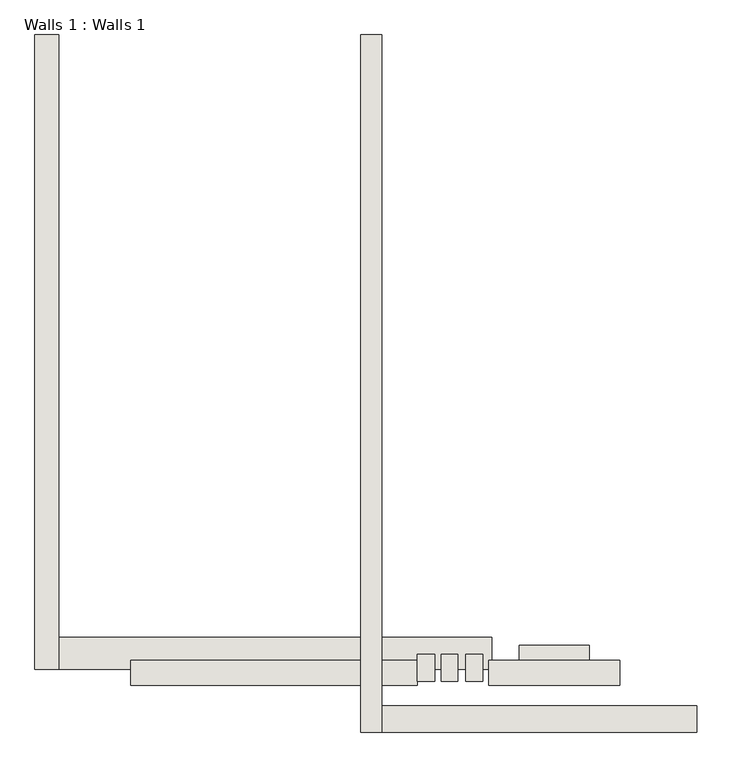
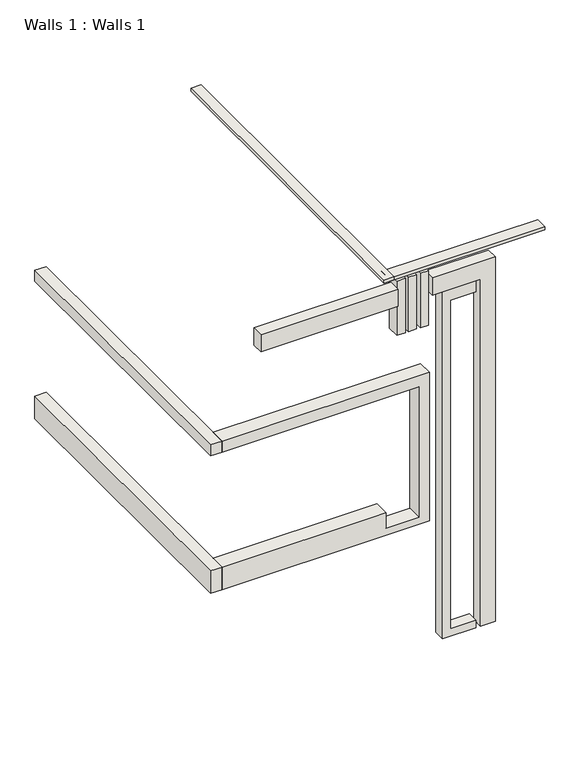
"""IFC4 building model written with IfcOpenShell, lengths in millimetres: wall geometry, Walls 1 : Walls 1."""

from ifc_helpers import new_model, si_unit, frame, origin, place, context, project, spatial, polyline, outline, extrude, source, transform, mapped, element, save


def walls_1_walls_1_d3114a13(model_context):
    return source(origin(), model_context, "Body", "SweptSolid", [
        extrude(outline(polyline([(-3875.3528989, 2861.5277146), (-3875.3528989, 11743.1483979), (-3610.0128864, 11743.1483979), (-3610.0128864, 2861.5277146), (-3875.3528989, 2861.5277146)])), frame((0.0, 0.0, 11198.7570873), z_axis=(0.0, 0.0, 1.0), x_axis=(1.0, 0.0, 0.0)), (0.0, 0.0, 1.0), 78.8429127),
        extrude(outline(polyline([(399.1874342, 2861.5277146), (-3753.7125658, 2861.5277146), (-3753.7125658, 3200.3867317), (399.1874342, 3200.3867317), (399.1874342, 2861.5277146)])), frame((0.0, 0.0, 11198.7570873), z_axis=(0.0, 0.0, 1.0), x_axis=(1.0, 0.0, 0.0)), (0.0, 0.0, 1.0), 78.8429127),
        extrude(outline(polyline([(-8020.9125658, 3665.9483979), (-8020.9125658, 11743.1483979), (-7716.1125658, 11743.1483979), (-7716.1125658, 3665.9483979), (-8020.9125658, 3665.9483979)])), frame((0.0, 0.0, 3454.4), z_axis=(0.0, 0.0, 1.0), x_axis=(1.0, 0.0, 0.0)), (0.0, 0.0, 1.0), 633.0046424),
        extrude(outline(polyline([(-8020.9125658, 3665.9483979), (-8020.9125658, 11743.1483979), (-7716.1125658, 11743.1483979), (-7716.1125658, 3665.9483979), (-8020.9125658, 3665.9483979)])), frame((0.0, 0.0, 7315.2), z_axis=(0.0, 0.0, 1.0), x_axis=(1.0, 0.0, 0.0)), (0.0, 0.0, 1.0), 304.8),
        extrude(outline(polyline([(7620.0, -2210.2300594), (7620.0, -7716.1125658), (7315.2, -7716.1125658), (7315.2, -2486.7301328), (3657.6, -2486.7301328), (3657.6, -3360.0125658), (4087.4046424, -3360.0125658), (4087.4046424, -7716.1125658), (3456.4466224, -7716.1125658), (3456.4466224, -3360.0125658), (3456.4466224, -2486.7301328), (3456.4466224, -2210.2300594), (7315.2, -2210.2300594), (7620.0, -2210.2300594)])), frame((0.0, 3665.9483979, 0.0), z_axis=(0.0, 1.0, 0.0), x_axis=(0.0, 0.0, 1.0)), (0.0, 0.0, 1.0), 406.4),
        extrude(outline(polyline([(9825.7154641, -967.2365478), (9825.7154641, -1856.2365478), (25.4, -1856.2365478), (25.4, -967.2365478), (228.6, -967.2365478), (228.6, -1645.5125658), (9444.7154641, -1645.5125658), (9444.7154641, -967.2365478), (9825.7154641, -967.2365478)])), frame((0.0, 3665.9483979, 0.0), z_axis=(0.0, 1.0, 0.0), x_axis=(0.0, 0.0, 1.0)), (0.0, 0.0, 1.0), 304.8),
        extrude(outline(polyline([(-2935.9394594, 3516.0647491), (-3156.8125658, 3516.0647491), (-3156.8125658, 3858.3105061), (-2935.9394594, 3858.3105061), (-2935.9394594, 3516.0647491)])), frame((0.0, 0.0, 9080.547311), z_axis=(0.0, 0.0, 1.0), x_axis=(1.0, 0.0, 0.0)), (0.0, 0.0, 1.0), 1524.0),
        extrude(outline(polyline([(-2639.4084614, 3516.0647491), (-2850.1955564, 3516.0647491), (-2850.1955564, 3858.3105061), (-2639.4084614, 3858.3105061), (-2639.4084614, 3516.0647491)])), frame((0.0, 0.0, 9080.547311), z_axis=(0.0, 0.0, 1.0), x_axis=(1.0, 0.0, 0.0)), (0.0, 0.0, 1.0), 1524.0),
        extrude(outline(polyline([(-2325.0141503, 3516.0647491), (-2535.8012452, 3516.0647491), (-2535.8012452, 3858.3105061), (-2325.0141503, 3858.3105061), (-2325.0141503, 3516.0647491)])), frame((0.0, 0.0, 9080.547311), z_axis=(0.0, 0.0, 1.0), x_axis=(1.0, 0.0, 0.0)), (0.0, 0.0, 1.0), 1524.0),
        extrude(outline(polyline([(-3156.8125658, 3463.0052053), (-6801.7125658, 3463.0052053), (-6801.7125658, 3780.2263443), (-3156.8125658, 3780.2263443), (-3156.8125658, 3463.0052053)])), frame((0.0, 0.0, 9927.3154641), z_axis=(0.0, 0.0, 1.0), x_axis=(1.0, 0.0, 0.0)), (0.0, 0.0, 1.0), 486.6845359),
        extrude(outline(polyline([(10058.4, -576.9943988), (10414.0, -576.9943988), (10414.0, -2246.8128437), (9927.3154641, -2246.8128437), (9927.3154641, -967.2365478), (187.1567832, -967.2365478), (187.1567832, -576.9943988), (10058.4, -576.9943988)])), frame((0.0, 3463.0052053, 0.0), z_axis=(0.0, 1.0, 0.0), x_axis=(0.0, 0.0, 1.0)), (0.0, 0.0, 1.0), 317.221139),
    ])


if __name__ == "__main__":
    model = new_model("IFC4")
    model_context = context("Model", 3, world=origin())
    ifc_project = project(units=[si_unit("LENGTHUNIT", "METRE", prefix="MILLI")], contexts=[model_context])
    site = spatial("IfcSite", under=ifc_project)
    building = spatial("IfcBuilding", under=site)
    placement = place(None, origin())
    walls_1_walls_1_shape = walls_1_walls_1_d3114a13(model_context)
    element("IfcWall", 1, ObjectType="Walls 1 : Walls 1", at=placement, inside=building, context=model_context, shape_type="MappedRepresentation", body=[
        mapped(walls_1_walls_1_shape, transform((0.0, 0.0, 0.0), x_axis=(1.0, 0.0, 0.0), y_axis=(0.0, 1.0, 0.0), z_axis=(0.0, 0.0, 1.0))),
    ])
    save(model, "model.ifc")

# Revit data of these elements
# Element 1 (IfcWall, "Walls 1 : Walls 1")
#   Materials on its faces: "Default Wall"
# Materials
#   "Default Wall": colour RGB 128 128 128, transparency 0
